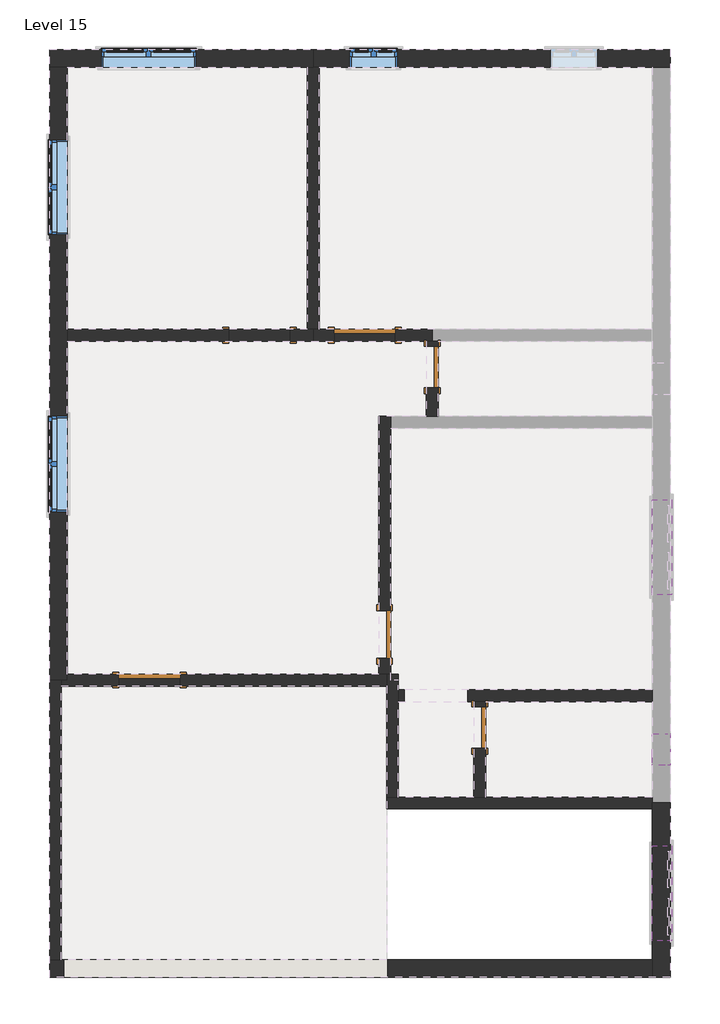
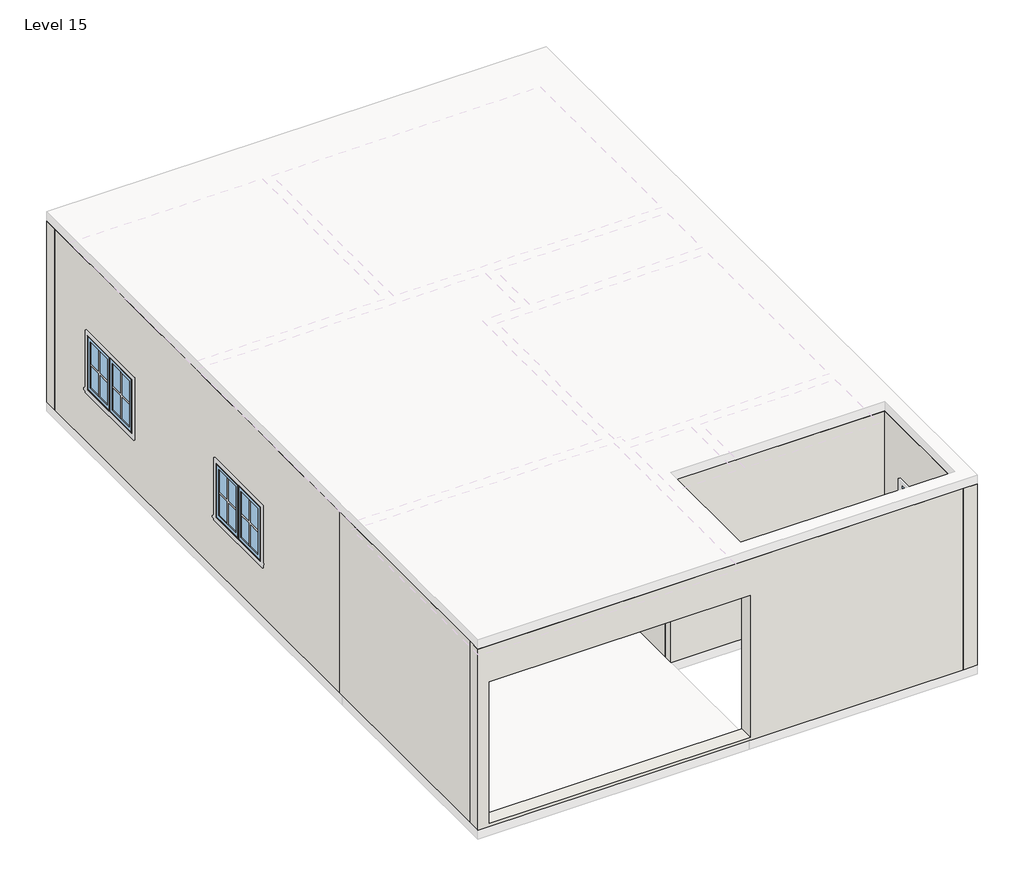
# One storey, part 1 of 2: 24 walls, 10 windows, 6 doors.
"""IFC4 building model written with IfcOpenShell, lengths in millimetres."""

from ifc_helpers import new_model, si_unit, frame, origin, place, context, project, spatial, polyline, outline, extrude, faceted_brep, transform, mapped, element, save
from components import door_2908be75, door_9ea4ff49, door_dc34e247, door_b804d09e, fixed_2_415b3208, window_casement_double_3_c417fced, window_casement_double_4_c19c33cb

model = new_model("IFC4")

# Units and contexts
model_context = context("Model", 3, world=origin())
ifc_project = project(units=[si_unit("LENGTHUNIT", "METRE", prefix="MILLI")], contexts=[model_context])

# Site, building, storey
site = spatial("IfcSite", under=ifc_project)
building = spatial("IfcBuilding", under=site)
storey = spatial("IfcBuildingStorey", under=building, Name="Level 15", Elevation=6400.8)

# Doors
placement = place(None, origin())
door_shape = door_2908be75(model_context)
element("IfcDoor", 1, ObjectType="Single-Flush : 1' 9\"", at=placement, inside=storey, context=model_context, shape_type="MappedRepresentation", body=[
    mapped(door_shape, transform((-397.3154463, -2781.5544725, 6400.8), x_axis=(0.0, 1.0, 0.0), y_axis=(-1.0, 0.0, 0.0), z_axis=(0.0, 0.0, 1.0))),
])
element("IfcDoor", 2, ObjectType="Single-Flush : 1' 9\"", at=placement, inside=storey, context=model_context, shape_type="MappedRepresentation", body=[
    mapped(door_shape, transform((-1006.9154463, 1841.2455275, 6400.8), x_axis=(0.0, 1.0, 0.0), y_axis=(-1.0, 0.0, 0.0), z_axis=(0.0, 0.0, 1.0))),
])
door_2_shape = door_9ea4ff49(model_context)
element("IfcDoor", 3, ObjectType="Single-Flush : 2'0\"", at=placement, inside=storey, context=model_context, shape_type="MappedRepresentation", body=[
    mapped(door_2_shape, transform((-1616.5154463, -1587.7544725, 6400.8), x_axis=(0.0, -1.0, 0.0), y_axis=(1.0, 0.0, 0.0), z_axis=(0.0, 0.0, 1.0))),
])
door_3_shape = door_dc34e247(model_context)
element("IfcDoor", 4, ObjectType="Single-Flush : 2'7\"", at=placement, inside=storey, context=model_context, shape_type="MappedRepresentation", body=[
    mapped(door_3_shape, transform((-4626.4154463, -2171.9544725, 6400.8), x_axis=(-1.0, 0.0, 0.0), y_axis=(0.0, -1.0, 0.0), z_axis=(0.0, 0.0, 1.0))),
])
element("IfcDoor", 5, ObjectType="Single-Flush : 2'7\"", at=placement, inside=storey, context=model_context, shape_type="MappedRepresentation", body=[
    mapped(door_3_shape, transform((-1870.5154463, 2247.6455275, 6400.8), x_axis=(-1.0, 0.0, 0.0), y_axis=(0.0, -1.0, 0.0), z_axis=(0.0, 0.0, 1.0))),
])
door_4_shape = door_b804d09e(model_context)
element("IfcDoor", 6, ObjectType="Single-Flush : 2'7\"", at=placement, inside=storey, context=model_context, shape_type="MappedRepresentation", body=[
    mapped(door_4_shape, transform((-3216.7154463, 2247.6455275, 6400.8), x_axis=(1.0, 0.0, 0.0), y_axis=(0.0, 1.0, 0.0), z_axis=(0.0, 0.0, 1.0))),
])

# Walls
element("IfcWall", 7, ObjectType="Generic - 6\"", at=placement, inside=storey, context=model_context, shape_type="Brep", body=[
    faceted_brep([(-5909.1154463, -2171.9544725, 6400.8), (-5909.1154463, -5753.3544725, 6400.8), (-5909.1154463, -5753.3544725, 9448.8), (-5909.1154463, -2171.9544725, 9448.8), (-5756.7154463, -2171.9544725, 6400.8), (-5756.7154463, -2171.9544725, 9448.8), (-5756.7154463, -2248.1544725, 9448.8), (-5756.7154463, -5753.3544725, 9448.8), (-5756.7154463, -5753.3544725, 6400.8), (-5756.7154463, -2248.1544725, 6400.8)], [[[0, 1, 2, 3]], [[4, 5, 6, 7, 8, 9]], [[1, 0, 4, 9, 8]], [[3, 2, 7, 6, 5]], [[0, 3, 5, 4]], [[2, 1, 8, 7]]]),
])
element("IfcWall", 8, ObjectType="Generic - 6\"", at=placement, inside=storey, context=model_context, shape_type="Brep", body=[
    faceted_brep([(1812.4845537, -3670.5544725, 6400.8), (-321.1154463, -3670.5544725, 6400.8), (-473.5154463, -3670.5544725, 6400.8), (-1438.7154463, -3670.5544725, 6400.8), (-1591.1154463, -3670.5544725, 6400.8), (-1591.1154463, -3670.5544725, 9448.8), (-1438.7154463, -3670.5544725, 9448.8), (-473.5154463, -3670.5544725, 9448.8), (-321.1154463, -3670.5544725, 9448.8), (1812.4845537, -3670.5544725, 9448.8), (1812.4845537, -3822.9544725, 6400.8), (1812.4845537, -3822.9544725, 9448.8), (-1591.1154463, -3822.9544725, 9448.8), (-1591.1154463, -3822.9544725, 6400.8), (1812.4845537, -3746.7544725, 6400.8), (1812.4845537, -3746.7544725, 9448.8)], [[[0, 1, 2, 3, 4, 5, 6, 7, 8, 9]], [[10, 11, 12, 13]], [[4, 3, 2, 1, 0, 14, 10, 13]], [[9, 8, 7, 6, 5, 12, 11, 15]], [[5, 4, 13, 12]], [[0, 9, 15, 11, 10, 14]]]),
])
element("IfcWall", 9, ObjectType="Generic - 6\"", at=placement, inside=storey, context=model_context, shape_type="Brep", body=[
    faceted_brep([(-1438.7154463, -3670.5544725, 6400.8), (-1438.7154463, -2451.3544725, 6400.8), (-1438.7154463, -2298.9544725, 6400.8), (-1438.7154463, -2095.7544725, 6400.8), (-1438.7154463, -2095.7544725, 9448.8), (-1438.7154463, -2298.9544725, 9448.8), (-1438.7154463, -2451.3544725, 9448.8), (-1438.7154463, -3670.5544725, 9448.8), (-1591.1154463, -3670.5544725, 6400.8), (-1591.1154463, -3670.5544725, 9448.8), (-1591.1154463, -2248.1544725, 9448.8), (-1591.1154463, -2171.9544725, 9448.8), (-1591.1154463, -2095.7544725, 9448.8), (-1591.1154463, -2095.7544725, 6400.8), (-1591.1154463, -2171.9544725, 6400.8), (-1591.1154463, -2248.1544725, 6400.8), (-1540.3154463, -2095.7544725, 6400.8), (-1540.3154463, -2095.7544725, 9448.8)], [[[0, 1, 2, 3, 4, 5, 6, 7]], [[8, 9, 10, 11, 12, 13, 14, 15]], [[3, 2, 1, 0, 8, 15, 14, 13, 16]], [[7, 6, 5, 4, 17, 12, 11, 10, 9]], [[0, 7, 9, 8]], [[4, 3, 16, 13, 12, 17]]]),
])
element("IfcWall", 10, ObjectType="Generic - 6\"", at=placement, inside=storey, context=model_context, shape_type="Brep", body=[
    faceted_brep([(-5020.1154463, -2095.7544725, 8534.4), (-5020.1154463, -2095.7544725, 6400.8), (-5680.5154463, -2095.7544725, 6400.8), (-5680.5154463, -2095.7544725, 9448.8), (-1692.7154463, -2095.7544725, 9448.8), (-1591.1154463, -2095.7544725, 9448.8), (-1591.1154463, -2095.7544725, 6400.8), (-1692.7154463, -2095.7544725, 6400.8), (-4232.7154463, -2095.7544725, 6400.8), (-4232.7154463, -2095.7544725, 8534.4), (-5756.7154463, -2248.1544725, 6400.8), (-5020.1154463, -2248.1544725, 6400.8), (-5020.1154463, -2248.1544725, 8534.4), (-4232.7154463, -2248.1544725, 8534.4), (-4232.7154463, -2248.1544725, 6400.8), (-1591.1154463, -2248.1544725, 6400.8), (-1591.1154463, -2248.1544725, 9448.8), (-5756.7154463, -2248.1544725, 9448.8), (-5756.7154463, -2171.9544725, 6400.8), (-5680.5154463, -2171.9544725, 6400.8), (-5680.5154463, -2171.9544725, 9448.8), (-5756.7154463, -2171.9544725, 9448.8)], [[[0, 1, 2, 3, 4, 5, 6, 7, 8, 9]], [[10, 11, 12, 13, 14, 15, 16, 17]], [[2, 1, 11, 10, 18, 19]], [[8, 7, 6, 15, 14]], [[5, 4, 3, 20, 21, 17, 16]], [[3, 2, 19, 20]], [[19, 18, 21, 20]], [[18, 10, 17, 21]], [[6, 5, 16, 15]], [[12, 11, 1, 0]], [[13, 12, 0, 9]], [[14, 13, 9, 8]]]),
])
element("IfcWall", 11, ObjectType="Generic - 6\"", at=placement, inside=storey, context=model_context, shape_type="Brep", body=[
    faceted_brep([(1812.4845537, -2451.3544725, 6400.8), (1812.4845537, -2451.3544725, 9448.8), (-321.1154463, -2451.3544725, 9448.8), (-473.5154463, -2451.3544725, 9448.8), (-1438.7154463, -2451.3544725, 9448.8), (-1438.7154463, -2451.3544725, 6400.8), (-1367.0206652, -2451.3544725, 6400.8), (-1367.0206652, -2451.3544725, 8839.2), (-547.4818767, -2451.3544725, 8839.2), (-547.4818767, -2451.3544725, 6400.8), (-473.5154463, -2451.3544725, 6400.8), (-321.1154463, -2451.3544725, 6400.8), (1812.4845537, -2298.9544725, 9448.8), (1812.4845537, -2298.9544725, 6400.8), (-547.4818767, -2298.9544725, 6400.8), (-547.4818767, -2298.9544725, 8839.2), (-1367.0206652, -2298.9544725, 8839.2), (-1367.0206652, -2298.9544725, 6400.8), (-1438.7154463, -2298.9544725, 6400.8), (-1438.7154463, -2298.9544725, 9448.8)], [[[0, 1, 2, 3, 4, 5, 6, 7, 8, 9, 10, 11]], [[12, 13, 14, 15, 16, 17, 18, 19]], [[5, 18, 17, 6]], [[13, 0, 11, 10, 9, 14]], [[4, 3, 2, 1, 12, 19]], [[1, 0, 13, 12]], [[5, 4, 19, 18]], [[7, 16, 15, 8]], [[16, 7, 6, 17]], [[8, 15, 14, 9]]]),
])
element("IfcWall", 12, ObjectType="Generic - 6\"", at=placement, inside=storey, context=model_context, shape_type="SweptSolid", body=[
    extrude(outline(polyline([(-2451.3544725, 6400.8), (-2514.8544725, 6400.8), (-2514.8544725, 8534.4), (-3048.2544725, 8534.4), (-3048.2544725, 6400.8), (-3670.5544725, 6400.8), (-3670.5544725, 9448.8), (-2451.3544725, 9448.8), (-2451.3544725, 6400.8)])), frame((-473.5154463, 0.0, 0.0), z_axis=(1.0, 0.0, 0.0), x_axis=(0.0, 1.0, 0.0)), (0.0, 0.0, 1.0), 152.4),
])
element("IfcWall", 13, ObjectType="Generic - 6\"", at=placement, inside=storey, context=model_context, shape_type="Brep", body=[
    faceted_brep([(-1540.3154463, -2095.7544725, 6400.8), (-1540.3154463, -1892.5544725, 6400.8), (-1540.3154463, -1892.5544725, 8534.4), (-1540.3154463, -1282.9544725, 8534.4), (-1540.3154463, -1282.9544725, 6400.8), (-1540.3154463, 1053.8455275, 6400.8), (-1540.3154463, 1206.2455275, 6400.8), (-1540.3154463, 1206.2455275, 9448.8), (-1540.3154463, 1053.8455275, 9448.8), (-1540.3154463, -2095.7544725, 9448.8), (-1692.7154463, -1892.5544725, 8534.4), (-1692.7154463, -1892.5544725, 6400.8), (-1692.7154463, -2095.7544725, 6400.8), (-1692.7154463, -2095.7544725, 9448.8), (-1692.7154463, 1206.2455275, 9448.8), (-1692.7154463, 1206.2455275, 6400.8), (-1692.7154463, -1282.9544725, 6400.8), (-1692.7154463, -1282.9544725, 8534.4), (-1591.1154463, -2095.7544725, 6400.8), (-1591.1154463, -2095.7544725, 9448.8)], [[[0, 1, 2, 3, 4, 5, 6, 7, 8, 9]], [[10, 11, 12, 13, 14, 15, 16, 17]], [[16, 15, 6, 5, 4]], [[12, 11, 1, 0, 18]], [[9, 8, 7, 14, 13, 19]], [[0, 9, 19, 13, 12, 18]], [[7, 6, 15, 14]], [[2, 1, 11, 10]], [[3, 2, 10, 17]], [[4, 3, 17, 16]]]),
])
element("IfcWall", 14, ObjectType="Generic - 6\"", at=placement, inside=storey, context=model_context, shape_type="Brep", body=[
    faceted_brep([(-930.7154463, 2107.9455275, 8534.4), (-930.7154463, 2107.9455275, 6400.8), (-930.7154463, 2171.4455275, 6400.8), (-930.7154463, 2171.4455275, 9448.8), (-930.7154463, 1206.2455275, 9448.8), (-930.7154463, 1206.2455275, 6400.8), (-930.7154463, 1574.5455275, 6400.8), (-930.7154463, 1574.5455275, 8534.4), (-1083.1154463, 2171.4455275, 6400.8), (-1083.1154463, 2107.9455275, 6400.8), (-1083.1154463, 2107.9455275, 8534.4), (-1083.1154463, 1574.5455275, 8534.4), (-1083.1154463, 1574.5455275, 6400.8), (-1083.1154463, 1206.2455275, 6400.8), (-1083.1154463, 1206.2455275, 9448.8), (-1083.1154463, 2171.4455275, 9448.8), (-1006.9154463, 2171.4455275, 6400.8), (-1006.9154463, 2171.4455275, 9448.8)], [[[0, 1, 2, 3, 4, 5, 6, 7]], [[8, 9, 10, 11, 12, 13, 14, 15]], [[6, 5, 13, 12]], [[2, 1, 9, 8, 16]], [[4, 3, 17, 15, 14]], [[5, 4, 14, 13]], [[10, 9, 1, 0]], [[11, 10, 0, 7]], [[12, 11, 7, 6]], [[3, 2, 16, 8, 15, 17]]]),
])
element("IfcWall", 15, ObjectType="Generic - 6\"", at=placement, inside=storey, context=model_context, shape_type="Brep", body=[
    faceted_brep([(-2607.1154463, 5678.2330275, 6400.8), (-2607.1154463, 2323.8455275, 6400.8), (-2607.1154463, 2323.8455275, 9448.8), (-2607.1154463, 5678.2330275, 9448.8), (-2454.7154463, 5678.2330275, 6400.8), (-2454.7154463, 5678.2330275, 9448.8), (-2454.7154463, 2323.8455275, 9448.8), (-2454.7154463, 2323.8455275, 6400.8), (-2530.9154463, 5678.2330275, 6400.8), (-2530.9154463, 2323.8455275, 6400.8), (-2530.9154463, 2323.8455275, 9448.8), (-2530.9154463, 5678.2330275, 9448.8)], [[[0, 1, 2, 3]], [[4, 5, 6, 7]], [[1, 0, 8, 4, 7, 9]], [[3, 2, 10, 6, 5, 11]], [[0, 3, 11, 5, 4, 8]], [[2, 1, 9, 7, 6, 10]]]),
])
element("IfcWall", 16, ObjectType="Generic - 6\"", at=placement, inside=storey, context=model_context, shape_type="Brep", body=[
    faceted_brep([(-2530.9154463, 2323.8455275, 6400.8), (-2607.1154463, 2323.8455275, 6400.8), (-2823.0154463, 2323.8455275, 6400.8), (-2823.0154463, 2323.8455275, 8534.4), (-3610.4154463, 2323.8455275, 8534.4), (-3610.4154463, 2323.8455275, 6400.8), (-5680.5154463, 2323.8455275, 6400.8), (-5680.5154463, 2323.8455275, 9448.8), (-2607.1154463, 2323.8455275, 9448.8), (-2530.9154463, 2323.8455275, 9448.8), (-2823.0154463, 2171.4455275, 8534.4), (-2823.0154463, 2171.4455275, 6400.8), (-2530.9154463, 2171.4455275, 6400.8), (-2530.9154463, 2171.4455275, 9448.8), (-5680.5154463, 2171.4455275, 9448.8), (-5680.5154463, 2171.4455275, 6400.8), (-3610.4154463, 2171.4455275, 6400.8), (-3610.4154463, 2171.4455275, 8534.4)], [[[0, 1, 2, 3, 4, 5, 6, 7, 8, 9]], [[10, 11, 12, 13, 14, 15, 16, 17]], [[16, 15, 6, 5]], [[12, 11, 2, 1, 0]], [[9, 8, 7, 14, 13]], [[0, 9, 13, 12]], [[7, 6, 15, 14]], [[5, 4, 17, 16]], [[4, 3, 10, 17]], [[3, 2, 11, 10]]]),
])
element("IfcWall", 17, ObjectType="Generic - 6\"", at=placement, inside=storey, context=model_context, shape_type="Brep", body=[
    faceted_brep([(-2264.2154463, 2323.8455275, 8534.4), (-2264.2154463, 2323.8455275, 6400.8), (-2454.7154463, 2323.8455275, 6400.8), (-2530.9154463, 2323.8455275, 6400.8), (-2530.9154463, 2323.8455275, 9448.8), (-2454.7154463, 2323.8455275, 9448.8), (-1006.9154463, 2323.8455275, 9448.8), (-1006.9154463, 2323.8455275, 6400.8), (-1476.8154463, 2323.8455275, 6400.8), (-1476.8154463, 2323.8455275, 8534.4), (-2530.9154463, 2171.4455275, 6400.8), (-2264.2154463, 2171.4455275, 6400.8), (-2264.2154463, 2171.4455275, 8534.4), (-1476.8154463, 2171.4455275, 8534.4), (-1476.8154463, 2171.4455275, 6400.8), (-1083.1154463, 2171.4455275, 6400.8), (-1006.9154463, 2171.4455275, 6400.8), (-1006.9154463, 2171.4455275, 9448.8), (-1083.1154463, 2171.4455275, 9448.8), (-2530.9154463, 2171.4455275, 9448.8)], [[[0, 1, 2, 3, 4, 5, 6, 7, 8, 9]], [[10, 11, 12, 13, 14, 15, 16, 17, 18, 19]], [[8, 7, 16, 15, 14]], [[3, 2, 1, 11, 10]], [[4, 3, 10, 19]], [[6, 5, 4, 19, 18, 17]], [[7, 6, 17, 16]], [[14, 13, 9, 8]], [[13, 12, 0, 9]], [[12, 11, 1, 0]]]),
])
element("IfcWall", 18, ObjectType="Generic - 6\"", at=placement, inside=storey, context=model_context, shape_type="SweptSolid", body=[
    extrude(outline(polyline([(-5680.5154463, -2095.7544725), (-1692.7154463, -2095.7544725), (-1692.7154463, -2171.9544725), (-1591.1154463, -2171.9544725), (-1591.1154463, -2248.1544725), (-5756.7154463, -2248.1544725), (-5756.7154463, -2171.9544725), (-5680.5154463, -2171.9544725), (-5680.5154463, -2095.7544725)])), frame((0.0, 0.0, 6400.8), z_axis=(0.0, 0.0, 1.0), x_axis=(1.0, 0.0, 0.0)), (0.0, 0.0, 1.0), 3048.0),
])
element("IfcWall", 19, ObjectType="Generic - 6\"", at=placement, inside=storey, context=model_context, shape_type="Brep", body=[
    faceted_brep([(-2607.1154463, 5678.2330275, 6400.8), (-2607.1154463, 2323.8455275, 6400.8), (-2607.1154463, 2323.8455275, 9448.8), (-2607.1154463, 5678.2330275, 9448.8), (-2454.7154463, 5678.2330275, 6400.8), (-2454.7154463, 5678.2330275, 9448.8), (-2454.7154463, 2323.8455275, 9448.8), (-2454.7154463, 2323.8455275, 6400.8), (-2530.9154463, 5678.2330275, 6400.8), (-2530.9154463, 2323.8455275, 6400.8), (-2530.9154463, 2323.8455275, 9448.8), (-2530.9154463, 5678.2330275, 9448.8)], [[[0, 1, 2, 3]], [[4, 5, 6, 7]], [[1, 0, 8, 4, 7, 9]], [[3, 2, 10, 6, 5, 11]], [[0, 3, 11, 5, 4, 8]], [[2, 1, 9, 7, 6, 10]]]),
])
element("IfcWall", 20, ObjectType="Generic - 6\"", at=placement, inside=storey, context=model_context, shape_type="Brep", body=[
    faceted_brep([(-2530.9154463, 2323.8455275, 6400.8), (-2607.1154463, 2323.8455275, 6400.8), (-5680.5154463, 2323.8455275, 6400.8), (-5680.5154463, 2323.8455275, 9448.8), (-2607.1154463, 2323.8455275, 9448.8), (-2530.9154463, 2323.8455275, 9448.8), (-2530.9154463, 2171.4455275, 6400.8), (-2530.9154463, 2171.4455275, 9448.8), (-5680.5154463, 2171.4455275, 9448.8), (-5680.5154463, 2171.4455275, 6400.8)], [[[0, 1, 2, 3, 4, 5]], [[6, 7, 8, 9]], [[2, 1, 0, 6, 9]], [[5, 4, 3, 8, 7]], [[0, 5, 7, 6]], [[3, 2, 9, 8]]]),
])
element("IfcWall", 21, ObjectType="Generic - 6\"", at=placement, inside=storey, context=model_context, shape_type="Brep", body=[
    faceted_brep([(-1006.9154463, 2323.8455275, 6400.8), (-2454.7154463, 2323.8455275, 6400.8), (-2530.9154463, 2323.8455275, 6400.8), (-2530.9154463, 2323.8455275, 9448.8), (-2454.7154463, 2323.8455275, 9448.8), (-1006.9154463, 2323.8455275, 9448.8), (-1006.9154463, 2171.4455275, 6400.8), (-1006.9154463, 2171.4455275, 9448.8), (-1083.1154463, 2171.4455275, 9448.8), (-2530.9154463, 2171.4455275, 9448.8), (-2530.9154463, 2171.4455275, 6400.8), (-1083.1154463, 2171.4455275, 6400.8)], [[[0, 1, 2, 3, 4, 5]], [[6, 7, 8, 9, 10, 11]], [[2, 1, 0, 6, 11, 10]], [[3, 2, 10, 9]], [[5, 4, 3, 9, 8, 7]], [[0, 5, 7, 6]]]),
])
element("IfcWall", 22, ObjectType="Generic - 9\"", at=placement, inside=storey, context=model_context, shape_type="Brep", body=[
    faceted_brep([(-5909.1154463, 5678.2330275, 6400.8), (-5680.5154463, 5678.2330275, 6400.8), (-2607.1154463, 5678.2330275, 6400.8), (-2530.9154463, 5678.2330275, 6400.8), (-2530.9154463, 5678.2330275, 9448.8), (-2607.1154463, 5678.2330275, 9448.8), (-5680.5154463, 5678.2330275, 9448.8), (-5909.1154463, 5678.2330275, 9448.8), (-4029.5154463, 5678.2330275, 8229.6), (-4029.5154463, 5678.2330275, 7315.2), (-5248.7154463, 5678.2330275, 7315.2), (-5248.7154463, 5678.2330275, 8229.6), (-5909.1154463, 5906.8330275, 6400.8), (-5909.1154463, 5906.8330275, 9448.8), (-2530.9154463, 5906.8330275, 9448.8), (-2530.9154463, 5906.8330275, 6400.8), (-4029.5154463, 5906.8330275, 8229.6), (-5248.7154463, 5906.8330275, 8229.6), (-5248.7154463, 5906.8330275, 7315.2), (-4029.5154463, 5906.8330275, 7315.2)], [[[0, 1, 2, 3, 4, 5, 6, 7], [8, 9, 10, 11]], [[12, 13, 14, 15], [16, 17, 18, 19]], [[3, 2, 1, 0, 12, 15]], [[4, 3, 15, 14]], [[7, 6, 5, 4, 14, 13]], [[0, 7, 13, 12]], [[9, 8, 16, 19]], [[10, 9, 19, 18]], [[11, 10, 18, 17]], [[8, 11, 17, 16]]]),
])
element("IfcWall", 23, ObjectType="Generic - 9\"", at=placement, inside=storey, context=model_context, shape_type="Brep", body=[
    faceted_brep([(1812.4845537, -5753.3544725, 6400.8), (-5756.7154463, -5753.3544725, 6400.8), (-5909.1154463, -5753.3544725, 6400.8), (-5909.1154463, -5753.3544725, 9448.8), (-5756.7154463, -5753.3544725, 9448.8), (1812.4845537, -5753.3544725, 9448.8), (-1576.8982041, -5753.3544725, 8839.2), (-5729.1673724, -5753.3544725, 8839.2), (-5729.1673724, -5753.3544725, 6451.6), (-1576.8982041, -5753.3544725, 6451.6), (-5909.1154463, -5981.9544725, 6400.8), (1812.4845537, -5981.9544725, 6400.8), (1812.4845537, -5981.9544725, 9448.8), (-5909.1154463, -5981.9544725, 9448.8), (-5729.1673724, -5981.9544725, 8839.2), (-1576.8982041, -5981.9544725, 8839.2), (-1576.8982041, -5981.9544725, 6451.6), (-5729.1673724, -5981.9544725, 6451.6)], [[[0, 1, 2, 3, 4, 5], [6, 7, 8, 9]], [[10, 11, 12, 13], [14, 15, 16, 17]], [[2, 1, 0, 11, 10]], [[5, 4, 3, 13, 12]], [[0, 5, 12, 11]], [[6, 15, 14, 7]], [[8, 17, 16, 9]], [[15, 6, 9, 16]], [[7, 14, 17, 8]], [[3, 2, 10, 13]]]),
])
element("IfcWall", 24, ObjectType="Generic - 9\"", at=placement, inside=storey, context=model_context, shape_type="Brep", body=[
    faceted_brep([(-5909.1154463, 5678.2330275, 6400.8), (-5909.1154463, -2171.9544725, 6400.8), (-5909.1154463, -2171.9544725, 9448.8), (-5909.1154463, 5678.2330275, 9448.8), (-5909.1154463, 4751.1330275, 8229.6), (-5909.1154463, 3531.9330275, 8229.6), (-5909.1154463, 3531.9330275, 7315.2), (-5909.1154463, 4751.1330275, 7315.2), (-5909.1154463, 1206.2455275, 8229.6), (-5909.1154463, -12.9544725, 8229.6), (-5909.1154463, -12.9544725, 7315.2), (-5909.1154463, 1206.2455275, 7315.2), (-5680.5154463, 5678.2330275, 6400.8), (-5680.5154463, 5678.2330275, 9448.8), (-5680.5154463, 2323.8455275, 9448.8), (-5680.5154463, 2171.4455275, 9448.8), (-5680.5154463, -2095.7544725, 9448.8), (-5680.5154463, -2171.9544725, 9448.8), (-5680.5154463, -2171.9544725, 6400.8), (-5680.5154463, -2095.7544725, 6400.8), (-5680.5154463, 2171.4455275, 6400.8), (-5680.5154463, 2323.8455275, 6400.8), (-5680.5154463, 4751.1330275, 8229.6), (-5680.5154463, 4751.1330275, 7315.2), (-5680.5154463, 3531.9330275, 7315.2), (-5680.5154463, 3531.9330275, 8229.6), (-5680.5154463, 1206.2455275, 8229.6), (-5680.5154463, 1206.2455275, 7315.2), (-5680.5154463, -12.9544725, 7315.2), (-5680.5154463, -12.9544725, 8229.6), (-5756.7154463, -2171.9544725, 6400.8), (-5756.7154463, -2171.9544725, 9448.8)], [[[0, 1, 2, 3], [4, 5, 6, 7], [8, 9, 10, 11]], [[12, 13, 14, 15, 16, 17, 18, 19, 20, 21], [22, 23, 24, 25], [26, 27, 28, 29]], [[1, 0, 12, 21, 20, 19, 18, 30]], [[2, 1, 30, 18, 17, 31]], [[3, 2, 31, 17, 16, 15, 14, 13]], [[0, 3, 13, 12]], [[23, 22, 4, 7]], [[24, 23, 7, 6]], [[25, 24, 6, 5]], [[22, 25, 5, 4]], [[27, 26, 8, 11]], [[28, 27, 11, 10]], [[29, 28, 10, 9]], [[26, 29, 9, 8]]]),
])
element("IfcWall", 25, ObjectType="Generic - 9\"", at=placement, inside=storey, context=model_context, shape_type="Brep", body=[
    faceted_brep([(-2530.9154463, 5678.2330275, 6400.8), (-2454.7154463, 5678.2330275, 6400.8), (1812.4845537, 5678.2330275, 6400.8), (2041.0845537, 5678.2330275, 6400.8), (2041.0845537, 5678.2330275, 9448.8), (1812.4845537, 5678.2330275, 9448.8), (-2454.7154463, 5678.2330275, 9448.8), (-2530.9154463, 5678.2330275, 9448.8), (-1451.4154463, 5678.2330275, 8229.6), (-1451.4154463, 5678.2330275, 7315.2), (-2061.0154463, 5678.2330275, 7315.2), (-2061.0154463, 5678.2330275, 8229.6), (1113.9845537, 5678.2330275, 8229.6), (1113.9845537, 5678.2330275, 7315.2), (504.3845537, 5678.2330275, 7315.2), (504.3845537, 5678.2330275, 8229.6), (-2530.9154463, 5906.8330275, 6400.8), (-2530.9154463, 5906.8330275, 9448.8), (2041.0845537, 5906.8330275, 9448.8), (2041.0845537, 5906.8330275, 6400.8), (-1451.4154463, 5906.8330275, 8229.6), (-2061.0154463, 5906.8330275, 8229.6), (-2061.0154463, 5906.8330275, 7315.2), (-1451.4154463, 5906.8330275, 7315.2), (1113.9845537, 5906.8330275, 8229.6), (504.3845537, 5906.8330275, 8229.6), (504.3845537, 5906.8330275, 7315.2), (1113.9845537, 5906.8330275, 7315.2)], [[[0, 1, 2, 3, 4, 5, 6, 7], [8, 9, 10, 11], [12, 13, 14, 15]], [[16, 17, 18, 19], [20, 21, 22, 23], [24, 25, 26, 27]], [[3, 2, 1, 0, 16, 19]], [[7, 6, 5, 4, 18, 17]], [[0, 7, 17, 16]], [[4, 3, 19, 18]], [[8, 11, 21, 20]], [[11, 10, 22, 21]], [[10, 9, 23, 22]], [[9, 8, 20, 23]], [[12, 15, 25, 24]], [[15, 14, 26, 25]], [[14, 13, 27, 26]], [[13, 12, 24, 27]]]),
])
element("IfcWall", 26, ObjectType="Generic - 9\"", at=placement, inside=storey, context=model_context, shape_type="Brep", body=[
    faceted_brep([(1812.4845537, -3746.7544725, 6400.8), (1812.4845537, -3822.9544725, 6400.8), (1812.4845537, -5753.3544725, 6400.8), (1812.4845537, -5981.9544725, 6400.8), (1812.4845537, -5981.9544725, 9448.8), (1812.4845537, -5753.3544725, 9448.8), (1812.4845537, -3822.9544725, 9448.8), (1812.4845537, -3746.7544725, 9448.8), (1812.4845537, -5512.0544725, 8534.4), (1812.4845537, -5512.0544725, 7620.0), (1812.4845537, -4292.8544725, 7620.0), (1812.4845537, -4292.8544725, 8534.4), (2041.0845537, -3746.7544725, 6400.8), (2041.0845537, -3746.7544725, 9448.8), (2041.0845537, -5981.9544725, 9448.8), (2041.0845537, -5981.9544725, 6400.8), (2041.0845537, -5512.0544725, 8534.4), (2041.0845537, -4292.8544725, 8534.4), (2041.0845537, -4292.8544725, 7620.0), (2041.0845537, -5512.0544725, 7620.0)], [[[0, 1, 2, 3, 4, 5, 6, 7], [8, 9, 10, 11]], [[12, 13, 14, 15], [16, 17, 18, 19]], [[3, 2, 1, 0, 12, 15]], [[7, 6, 5, 4, 14, 13]], [[0, 7, 13, 12]], [[4, 3, 15, 14]], [[8, 11, 17, 16]], [[11, 10, 18, 17]], [[10, 9, 19, 18]], [[9, 8, 16, 19]]]),
])
element("IfcWall", 27, ObjectType="Generic - 9\"", at=placement, inside=storey, context=model_context, shape_type="SweptSolid", body=[
    extrude(outline(polyline([(6400.8, -5680.5154463), (6400.8, -2607.1154463), (9448.8, -2607.1154463), (9448.8, -5680.5154463), (6400.8, -5680.5154463)]), holes=[polyline([(8229.6, -4029.5154463), (7315.2, -4029.5154463), (7315.2, -5248.7154463), (8229.6, -5248.7154463), (8229.6, -4029.5154463)])]), frame((0.0, 5678.2330275, 0.0), z_axis=(0.0, 1.0, 0.0), x_axis=(0.0, 0.0, 1.0)), (0.0, 0.0, 1.0), 228.6),
])
element("IfcWall", 28, ObjectType="Generic - 9\"", at=placement, inside=storey, context=model_context, shape_type="Brep", body=[
    faceted_brep([(1812.4845537, -5753.3544725, 6400.8), (-5756.7154463, -5753.3544725, 6400.8), (-5909.1154463, -5753.3544725, 6400.8), (-5909.1154463, -5753.3544725, 9448.8), (-5756.7154463, -5753.3544725, 9448.8), (1812.4845537, -5753.3544725, 9448.8), (-1576.8982041, -5753.3544725, 8839.2), (-5729.1673724, -5753.3544725, 8839.2), (-5729.1673724, -5753.3544725, 6451.6), (-1576.8982041, -5753.3544725, 6451.6), (-5909.1154463, -5981.9544725, 6400.8), (1812.4845537, -5981.9544725, 6400.8), (1812.4845537, -5981.9544725, 9448.8), (-5909.1154463, -5981.9544725, 9448.8), (-5729.1673724, -5981.9544725, 8839.2), (-1576.8982041, -5981.9544725, 8839.2), (-1576.8982041, -5981.9544725, 6451.6), (-5729.1673724, -5981.9544725, 6451.6)], [[[0, 1, 2, 3, 4, 5], [6, 7, 8, 9]], [[10, 11, 12, 13], [14, 15, 16, 17]], [[2, 1, 0, 11, 10]], [[5, 4, 3, 13, 12]], [[6, 15, 14, 7]], [[8, 17, 16, 9]], [[15, 6, 9, 16]], [[7, 14, 17, 8]], [[3, 2, 10, 13]], [[0, 5, 12, 11]]]),
])
element("IfcWall", 29, ObjectType="Generic - 9\"", at=placement, inside=storey, context=model_context, shape_type="SweptSolid", body=[
    extrude(outline(polyline([(6400.8, -2454.7154463), (6400.8, 1812.4845537), (9448.8, 1812.4845537), (9448.8, -2454.7154463), (6400.8, -2454.7154463)]), holes=[polyline([(8229.6, -1451.4154463), (7315.2, -1451.4154463), (7315.2, -2061.0154463), (8229.6, -2061.0154463), (8229.6, -1451.4154463)]), polyline([(8229.6, 1113.9845537), (7315.2, 1113.9845537), (7315.2, 504.3845537), (8229.6, 504.3845537), (8229.6, 1113.9845537)])]), frame((0.0, 5678.2330275, 0.0), z_axis=(0.0, 1.0, 0.0), x_axis=(0.0, 0.0, 1.0)), (0.0, 0.0, 1.0), 228.6),
])
element("IfcWall", 30, ObjectType="Generic - 9\"", at=placement, inside=storey, context=model_context, shape_type="SweptSolid", body=[
    extrude(outline(polyline([(-3822.9544725, 6400.8), (-5753.3544725, 6400.8), (-5753.3544725, 9448.8), (-3822.9544725, 9448.8), (-3822.9544725, 6400.8)]), holes=[polyline([(-5512.0544725, 8534.4), (-5512.0544725, 7620.0), (-4292.8544725, 7620.0), (-4292.8544725, 8534.4), (-5512.0544725, 8534.4)])]), frame((1812.4845537, 0.0, 0.0), z_axis=(1.0, 0.0, 0.0), x_axis=(0.0, 1.0, 0.0)), (0.0, 0.0, 1.0), 228.6),
])

# Windows
fixed_2_shape = fixed_2_415b3208(model_context)
element("IfcWindow", 31, ObjectType="Fixed : 2'", at=placement, inside=storey, context=model_context, shape_type="MappedRepresentation", body=[
    mapped(fixed_2_shape, transform((1926.7845537, -3099.0544725, 7924.8), x_axis=(0.0, -1.0, 0.0), y_axis=(1.0, 0.0, 0.0), z_axis=(0.0, 0.0, 1.0))),
])
window_casement_double_3_shape = window_casement_double_3_c417fced(model_context)
element("IfcWindow", 32, ObjectType="Window-Casement-Double : 3'", at=placement, inside=storey, context=model_context, shape_type="MappedRepresentation", body=[
    mapped(window_casement_double_3_shape, transform((-1756.2154463, 5792.5330275, 6400.8), x_axis=(1.0, 0.0, 0.0), y_axis=(0.0, 1.0, 0.0), z_axis=(0.0, 0.0, 1.0))),
])
element("IfcWindow", 33, ObjectType="Window-Casement-Double : 3'", at=placement, inside=storey, context=model_context, shape_type="MappedRepresentation", body=[
    mapped(window_casement_double_3_shape, transform((-1756.2154463, 5792.5330275, 6400.8), x_axis=(1.0, 0.0, 0.0), y_axis=(0.0, 1.0, 0.0), z_axis=(0.0, 0.0, 1.0))),
])
window_casement_double_4_shape = window_casement_double_4_c19c33cb(model_context)
element("IfcWindow", 34, ObjectType="Window-Casement-Double : 4'", at=placement, inside=storey, context=model_context, shape_type="MappedRepresentation", body=[
    mapped(window_casement_double_4_shape, transform((-4639.1154463, 5792.5330275, 6400.8), x_axis=(1.0, 0.0, 0.0), y_axis=(0.0, 1.0, 0.0), z_axis=(0.0, 0.0, 1.0))),
])
element("IfcWindow", 35, ObjectType="Window-Casement-Double : 4'", at=placement, inside=storey, context=model_context, shape_type="MappedRepresentation", body=[
    mapped(window_casement_double_4_shape, transform((-5794.8154463, 4141.5330275, 6400.8), x_axis=(0.0, 1.0, 0.0), y_axis=(-1.0, 0.0, 0.0), z_axis=(0.0, 0.0, 1.0))),
])
element("IfcWindow", 36, ObjectType="Window-Casement-Double : 4'", at=placement, inside=storey, context=model_context, shape_type="MappedRepresentation", body=[
    mapped(window_casement_double_4_shape, transform((-5794.8154463, 596.6455275, 6400.8), x_axis=(0.0, 1.0, 0.0), y_axis=(-1.0, 0.0, 0.0), z_axis=(0.0, 0.0, 1.0))),
])
element("IfcWindow", 37, ObjectType="Window-Casement-Double : 4'", at=placement, inside=storey, context=model_context, shape_type="MappedRepresentation", body=[
    mapped(window_casement_double_4_shape, transform((1926.7845537, -470.1544725, 6705.6), x_axis=(0.0, -1.0, 0.0), y_axis=(1.0, 0.0, 0.0), z_axis=(0.0, 0.0, 1.0))),
])
element("IfcWindow", 38, ObjectType="Window-Casement-Double : 4'", at=placement, inside=storey, context=model_context, shape_type="MappedRepresentation", body=[
    mapped(window_casement_double_4_shape, transform((1926.7845537, -4902.4544725, 6705.6), x_axis=(0.0, -1.0, 0.0), y_axis=(1.0, 0.0, 0.0), z_axis=(0.0, 0.0, 1.0))),
])
element("IfcWindow", 39, ObjectType="Window-Casement-Double : 4'", at=placement, inside=storey, context=model_context, shape_type="MappedRepresentation", body=[
    mapped(window_casement_double_4_shape, transform((-4639.1154463, 5792.5330275, 6400.8), x_axis=(1.0, 0.0, 0.0), y_axis=(0.0, 1.0, 0.0), z_axis=(0.0, 0.0, 1.0))),
])
element("IfcWindow", 40, ObjectType="Window-Casement-Double : 4'", at=placement, inside=storey, context=model_context, shape_type="MappedRepresentation", body=[
    mapped(window_casement_double_4_shape, transform((1926.7845537, -4902.4544725, 6705.6), x_axis=(0.0, -1.0, 0.0), y_axis=(1.0, 0.0, 0.0), z_axis=(0.0, 0.0, 1.0))),
])

save(model, "model.ifc")

# Revit data of these elements
# Type "Single-Flush : 1' 9\""
#   Type Mark = "10"
#   Construction Type Id = "MDOOR"
#   Assembly Code = "C1020"
#   Analytic Construction = "Metal"
#   Thickness = 0' - 2"
#   Heat Transfer Coefficient (U) = 0.651978 BTU/(h·ft²·°F)
#   Height = 7' - 0"
#   Trim Projection Ext = 0' - 1"
#   Trim Projection Int = 0' - 1"
#   Trim Width = 0' - 3"
#   Width = 1' - 9"
#   Define Thermal Properties by = 1
#   Door Material = Door - Panel
#   Frame Material = Door - Frame
#   Visual Light Transmittance = 0
#   Solar Heat Gain Coefficient = 0
#   Function = (empty or 0)
#   Wall Closure = (empty or 0)
# Type "Single-Flush : 2'0\""
#   Type Mark = "9"
#   Construction Type Id = "MDOOR"
#   Assembly Code = "C1020"
#   Analytic Construction = "Metal"
#   Thickness = 0' - 2"
#   Heat Transfer Coefficient (U) = 0.651978 BTU/(h·ft²·°F)
#   Height = 7' - 0"
#   Trim Projection Ext = 0' - 1"
#   Trim Projection Int = 0' - 1"
#   Trim Width = 0' - 3"
#   Width = 2' - 0"
#   Define Thermal Properties by = 1
#   Door Material = Door - Panel
#   Frame Material = Door - Frame
#   Visual Light Transmittance = 0
#   Solar Heat Gain Coefficient = 0
#   Function = (empty or 0)
#   Wall Closure = (empty or 0)
# Type "Single-Flush : 2'7\""
#   Type Mark = "8"
#   Construction Type Id = "MDOOR"
#   Assembly Code = "C1020"
#   Analytic Construction = "Metal"
#   Thickness = 0' - 2"
#   Heat Transfer Coefficient (U) = 0.651978 BTU/(h·ft²·°F)
#   Height = 7' - 0"
#   Trim Projection Ext = 0' - 1"
#   Trim Projection Int = 0' - 1"
#   Trim Width = 0' - 3"
#   Width = 2' - 7"
#   Define Thermal Properties by = 1
#   Door Material = Door - Panel
#   Frame Material = Door - Frame
#   Visual Light Transmittance = 0
#   Solar Heat Gain Coefficient = 0
#   Function = (empty or 0)
#   Wall Closure = (empty or 0)
# Type "Generic - 6\""
#   Assembly Code = "B2010"
#   Layers, outside or top first: 0' - 6" no material (function 1)
# Type "Generic - 9\""
#   Assembly Code = "B2010"
#   Layers, outside or top first: 0' - 9" no material (function 1)
# Type "Fixed : 2'"
#   Type Mark = "20"
#   Construction Type Id = "GSP4R"
#   Assembly Code = "B2020100"
#   Analytic Construction = "1/8 in Pilkington single glazing"
#   Visual Light Transmittance = 0.9
#   Solar Heat Gain Coefficient = 0.78
#   Heat Transfer Coefficient (U) = 0.6496 BTU/(h·ft²·°F)
#   Height = 2' - 0"
#   Default Sill Height = 1' - 0"
#   Width = 1' - 4"
#   Window Inset = 0' - 0 3/4"
#   Define Thermal Properties by = 1
#   Glass Pane Material = Glass
#   Sash Material = Sash
#   Wall Closure = (empty or 0)
# Type "Window-Casement-Double : 3'"
#   Type Mark = "19"
#   Fire Rating = "0.5h"
#   Assembly Code = "B2020100"
#   Analytic Construction = "Double glazing - domestic"
#   Frame Extension [instance default] = 0' - 0 1/4"
#   Window Inset [instance default] = 0' - 0"
#   Wall Thickness [instance default] = 0' - 6"
#   Interior Wall Closure [instance default] = 0' - 2 1/4"
#   Half Width = 1' - 0"
#   Visual Light Transmittance = 0.81
#   Thermal Resistance (R) = 1.8146 (h·ft²·°F)/BTU
#   Solar Heat Gain Coefficient = 0.76
#   Rough Width = 2' - 0 1/2"
#   Rough Height = 3' - 0 1/2"
#   Height = 3' - 0"
#   Heat Transfer Coefficient (U) = 0.5511 BTU/(h·ft²·°F)
#   Exterior Wall Closure [instance default] = 0' - 1 1/4"
#   Extension Jamb [instance default] = 0' - 2 1/4"
#   Default Sill Height = 3' - 0"
#   Width = 2' - 0"
#   Muntin Visibility = yes
#   Interior Trim Visibility [instance default] = yes
#   Exterior Trim Visibility [instance default] = yes
#   Extension Jamb Visibility [instance default] = yes
#   Interior Trim Material = Wood - Stained
#   Muntin Pattern = Muntin Pattern_2x2 : Muntin Pattern_2x2
#   Interior Trim = Trim-Window-Interior-Flat : Picture Frame
#   Interior Frame Material = Wood - Stained
#   Glass Panel Material = Glass
#   Exterior Trim Material = Clad - White
#   Exterior Trim = Trim-Window-Exterior-Flat : with Sill
#   Exterior Frame Material = Clad - White
#   Wall Closure = (empty or 0)
# Type "Window-Casement-Double : 4'"
#   Type Mark = "18"
#   Fire Rating = "0.5h"
#   Assembly Code = "B2020100"
#   Analytic Construction = "Double glazing - domestic"
#   Frame Extension [instance default] = 0' - 0 1/4"
#   Window Inset [instance default] = 0' - 0"
#   Wall Thickness [instance default] = 0' - 6"
#   Interior Wall Closure [instance default] = 0' - 2 1/4"
#   Half Width = 2' - 0"
#   Visual Light Transmittance = 0.81
#   Thermal Resistance (R) = 1.8146 (h·ft²·°F)/BTU
#   Solar Heat Gain Coefficient = 0.76
#   Rough Width = 4' - 0 1/2"
#   Rough Height = 3' - 0 1/2"
#   Height = 3' - 0"
#   Heat Transfer Coefficient (U) = 0.5511 BTU/(h·ft²·°F)
#   Exterior Wall Closure [instance default] = 0' - 1 1/4"
#   Extension Jamb [instance default] = 0' - 2 1/4"
#   Default Sill Height = 3' - 0"
#   Width = 4' - 0"
#   Muntin Visibility = yes
#   Interior Trim Visibility [instance default] = yes
#   Exterior Trim Visibility [instance default] = yes
#   Extension Jamb Visibility [instance default] = yes
#   Interior Trim Material = Wood - Stained
#   Muntin Pattern = Muntin Pattern_2x2 : Muntin Pattern_2x2
#   Interior Trim = Trim-Window-Interior-Flat : Picture Frame
#   Interior Frame Material = Wood - Stained
#   Glass Panel Material = Glass
#   Exterior Trim Material = Clad - White
#   Exterior Trim = Trim-Window-Exterior-Flat : with Sill
#   Exterior Frame Material = Clad - White
#   Wall Closure = (empty or 0)
# Elements 1, 2 (IfcDoor, "Single-Flush : 1' 9\"")
#   Phase Created = New Construction
#   Materials on its faces: "Door - Frame", "Door - Panel"
# Element 3 (IfcDoor, "Single-Flush : 2'0\"")
#   Phase Created = New Construction
#   Materials on its faces: "Door - Frame", "Door - Panel"
# Elements 4, 5, 6 (IfcDoor, "Single-Flush : 2'7\"")
#   Phase Created = New Construction
#   Materials on its faces: "Door - Frame", "Door - Panel"
# Element 7 (IfcWall, "Generic - 6\"")
#   Top Offset = 0' - 0"
#   Base Offset = 0' - 0"
#   Unconnected Height = 10' - 0"
#   wall height = 10' - 0"
#   Phase Created = New Construction
#   Base Constraint = Level 15
#   Materials on its faces: "Default Wall", "WALL PAINT 4"
# Element 8 (IfcWall, "Generic - 6\"")
#   Top Offset = 0' - 0"
#   Base Offset = 0' - 0"
#   Unconnected Height = 10' - 0"
#   wall height = 10' - 0"
#   Phase Created = New Construction
#   Base Constraint = Level 15
#   Materials on its faces: "Default Wall", "MARBLE", "WALL PAINT 5"
# Element 9 (IfcWall, "Generic - 6\"")
#   Top Offset = 0' - 0"
#   Base Offset = 0' - 0"
#   Unconnected Height = 10' - 0"
#   wall height = 10' - 0"
#   Phase Created = New Construction
#   Base Constraint = Level 15
#   Materials on its faces: "Default Wall", "WALL PAINT 4", "MARBLE"
# Elements 10, 18 (IfcWall, "Generic - 6\"")
#   Top Offset = 0' - 0"
#   Base Offset = 0' - 0"
#   Unconnected Height = 10' - 0"
#   wall height = 10' - 0"
#   Phase Created = New Construction
#   Base Constraint = Level 15
#   Materials on its faces: "Default Wall", "WALL PAINT 2", "MARBLE"
# Element 11 (IfcWall, "Generic - 6\"")
#   Top Offset = 0' - 0"
#   Base Offset = 0' - 0"
#   Unconnected Height = 10' - 0"
#   wall height = 10' - 0"
#   Phase Created = New Construction
#   Base Constraint = Level 15
#   Materials on its faces: "Default Wall", "WALL PAINT 4", "WALL PAINT 5"
# Element 12 (IfcWall, "Generic - 6\"")
#   Top Offset = 0' - 0"
#   Base Offset = 0' - 0"
#   Unconnected Height = 10' - 0"
#   wall height = 10' - 0"
#   Phase Created = New Construction
#   Base Constraint = Level 15
#   Materials on its faces: "Default Wall", "WALL PAINT 5"
# Element 13 (IfcWall, "Generic - 6\"")
#   Top Offset = 0' - 0"
#   Base Offset = 0' - 0"
#   Unconnected Height = 10' - 0"
#   wall height = 10' - 0"
#   Phase Created = New Construction
#   Base Constraint = Level 15
#   Materials on its faces: "Default Wall", "WALL PAINT 4", "WALL PAINT 2", "WALL PAINT 5"
# Element 14 (IfcWall, "Generic - 6\"")
#   Top Offset = 0' - 0"
#   Base Offset = 0' - 0"
#   Unconnected Height = 10' - 0"
#   wall height = 10' - 0"
#   Phase Created = New Construction
#   Base Constraint = Level 15
#   Materials on its faces: "Default Wall", "WALL PAINT 5", "WALL PAINT 2"
# Elements 15, 19 (IfcWall, "Generic - 6\"")
#   Top Offset = 0' - 0"
#   Base Offset = 0' - 0"
#   Unconnected Height = 10' - 0"
#   wall height = 10' - 0"
#   Phase Created = New Construction
#   Base Constraint = Level 15
#   Materials on its faces: "Default Wall", "WALL PAINT 1", "WALL PAINT 3"
# Elements 16, 20 (IfcWall, "Generic - 6\"")
#   Top Offset = 0' - 0"
#   Base Offset = 0' - 0"
#   Unconnected Height = 10' - 0"
#   wall height = 10' - 0"
#   Phase Created = New Construction
#   Base Constraint = Level 15
#   Materials on its faces: "Default Wall", "WALL PAINT 1", "WALL PAINT 2"
# Elements 17, 21 (IfcWall, "Generic - 6\"")
#   Top Offset = 0' - 0"
#   Base Offset = 0' - 0"
#   Unconnected Height = 10' - 0"
#   wall height = 10' - 0"
#   Phase Created = New Construction
#   Base Constraint = Level 15
#   Materials on its faces: "Default Wall", "WALL PAINT 3", "WALL PAINT 2"
# Elements 22, 27 (IfcWall, "Generic - 9\"")
#   Top Offset = 0' - 0"
#   Base Offset = 0' - 0"
#   Unconnected Height = 10' - 0"
#   wall height = 10' - 0"
#   Phase Created = New Construction
#   Base Constraint = Level 15
#   Materials on its faces: "Default Wall", "WALL PAINT 1"
# Elements 23, 26, 28, 30 (IfcWall, "Generic - 9\"")
#   Top Offset = 0' - 0"
#   Base Offset = 0' - 0"
#   Unconnected Height = 10' - 0"
#   wall height = 10' - 0"
#   Phase Created = New Construction
#   Base Constraint = Level 15
#   Materials on its faces: "Default Wall", "WALL PAINT 4"
# Element 24 (IfcWall, "Generic - 9\"")
#   Top Offset = 0' - 0"
#   Base Offset = 0' - 0"
#   Unconnected Height = 10' - 0"
#   wall height = 10' - 0"
#   Phase Created = New Construction
#   Base Constraint = Level 15
#   Materials on its faces: "Default Wall"
# Elements 25, 29 (IfcWall, "Generic - 9\"")
#   Top Offset = 0' - 0"
#   Base Offset = 0' - 0"
#   Unconnected Height = 10' - 0"
#   wall height = 10' - 0"
#   Phase Created = New Construction
#   Base Constraint = Level 15
#   Materials on its faces: "Default Wall", "WALL PAINT 3"
# Element 31 (IfcWindow, "Fixed : 2'")
#   Mark = "47"
#   Phase Created = New Construction
#   Materials on its faces: "Sash", "Glass"
# Element 32 (IfcWindow, "Window-Casement-Double : 3'")
#   Mark = "45"
#   Window Inset = 0' - 0"
#   Interior Wall Closure = 0' - 2 1/4"
#   Frame Extension = 0' - 0 1/4"
#   Exterior Wall Closure = 0' - 1 1/4"
#   Interior Trim Visibility = yes
#   Exterior Trim Visibility = yes
#   Phase Created = New Construction
#   Materials on its faces: "Wood - Stained", "Glass", "Clad - White"
# Element 33 (IfcWindow, "Window-Casement-Double : 3'")
#   Mark = "51"
#   Window Inset = 0' - 0"
#   Interior Wall Closure = 0' - 2 1/4"
#   Frame Extension = 0' - 0 1/4"
#   Exterior Wall Closure = 0' - 1 1/4"
#   Interior Trim Visibility = yes
#   Exterior Trim Visibility = yes
#   Phase Created = New Construction
#   Materials on its faces: "Wood - Stained", "Glass", "Clad - White"
# Element 34 (IfcWindow, "Window-Casement-Double : 4'")
#   Mark = "40"
#   Window Inset = 0' - 0"
#   Interior Wall Closure = 0' - 2 1/4"
#   Frame Extension = 0' - 0 1/4"
#   Exterior Wall Closure = 0' - 1 1/4"
#   Interior Trim Visibility = yes
#   Exterior Trim Visibility = yes
#   Phase Created = New Construction
#   Materials on its faces: "Wood - Stained", "Glass", "Clad - White"
# Element 35 (IfcWindow, "Window-Casement-Double : 4'")
#   Mark = "41"
#   Window Inset = 0' - 0"
#   Interior Wall Closure = 0' - 2 1/4"
#   Frame Extension = 0' - 0 1/4"
#   Exterior Wall Closure = 0' - 1 1/4"
#   Interior Trim Visibility = yes
#   Exterior Trim Visibility = yes
#   Phase Created = New Construction
#   Materials on its faces: "Wood - Stained", "Glass", "Clad - White"
# Element 36 (IfcWindow, "Window-Casement-Double : 4'")
#   Mark = "42"
#   Window Inset = 0' - 0"
#   Interior Wall Closure = 0' - 2 1/4"
#   Frame Extension = 0' - 0 1/4"
#   Exterior Wall Closure = 0' - 1 1/4"
#   Interior Trim Visibility = yes
#   Exterior Trim Visibility = yes
#   Phase Created = New Construction
#   Materials on its faces: "Wood - Stained", "Glass", "Clad - White"
# Element 37 (IfcWindow, "Window-Casement-Double : 4'")
#   Mark = "43"
#   Window Inset = 0' - 0"
#   Interior Wall Closure = 0' - 2 1/4"
#   Frame Extension = 0' - 0 1/4"
#   Exterior Wall Closure = 0' - 1 1/4"
#   Interior Trim Visibility = yes
#   Exterior Trim Visibility = yes
#   Phase Created = New Construction
#   Materials on its faces: "Wood - Stained", "Glass", "Clad - White"
# Element 38 (IfcWindow, "Window-Casement-Double : 4'")
#   Mark = "44"
#   Window Inset = 0' - 0"
#   Interior Wall Closure = 0' - 2 1/4"
#   Frame Extension = 0' - 0 1/4"
#   Exterior Wall Closure = 0' - 1 1/4"
#   Interior Trim Visibility = yes
#   Exterior Trim Visibility = yes
#   Phase Created = New Construction
#   Materials on its faces: "Wood - Stained", "Glass", "Clad - White"
# Element 39 (IfcWindow, "Window-Casement-Double : 4'")
#   Mark = "49"
#   Window Inset = 0' - 0"
#   Interior Wall Closure = 0' - 2 1/4"
#   Frame Extension = 0' - 0 1/4"
#   Exterior Wall Closure = 0' - 1 1/4"
#   Interior Trim Visibility = yes
#   Exterior Trim Visibility = yes
#   Phase Created = New Construction
#   Materials on its faces: "Wood - Stained", "Glass", "Clad - White"
# Element 40 (IfcWindow, "Window-Casement-Double : 4'")
#   Mark = "50"
#   Window Inset = 0' - 0"
#   Interior Wall Closure = 0' - 2 1/4"
#   Frame Extension = 0' - 0 1/4"
#   Exterior Wall Closure = 0' - 1 1/4"
#   Interior Trim Visibility = yes
#   Exterior Trim Visibility = yes
#   Phase Created = New Construction
#   Materials on its faces: "Wood - Stained", "Glass", "Clad - White"
# Materials
#   "Door - Panel": class "Wood", colour RGB 210 159 95, transparency 0, Cost = 0
#   "Door - Frame": colour RGB 118 70 51, transparency 0, Cost = 0
#   "Glass": class "Glass", colour RGB 0 128 192, transparency 0.75, Description = "Soda Lime Glass", Cost = 0
#   "Sash": class "Wood", colour RGB 224 178 126, transparency 0, Cost = 0
#   "Wood - Stained": class "Wood", colour RGB 224 178 126, transparency 0, Cost = 0
#   "Clad - White": class "Wood", colour RGB 242 242 238, transparency 0, Cost = 0
#   "Default Wall": colour RGB 128 128 128, transparency 0, Cost = 0
#   "WALL PAINT 4": class "Generic", colour RGB 120 120 120, transparency 0, Cost = 0
#   "MARBLE": class "Generic", colour RGB 120 120 120, transparency 0, Cost = 0
#   "WALL PAINT 5": class "Generic", colour RGB 120 120 120, transparency 0, Cost = 0
#   "WALL PAINT 2": class "Generic", colour RGB 120 120 120, transparency 0, Cost = 0
#   "WALL PAINT 1": class "Generic", colour RGB 120 120 120, transparency 0, Cost = 0
#   "WALL PAINT 3": class "Generic", colour RGB 120 120 120, transparency 0, Cost = 0
